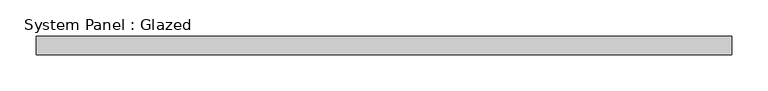
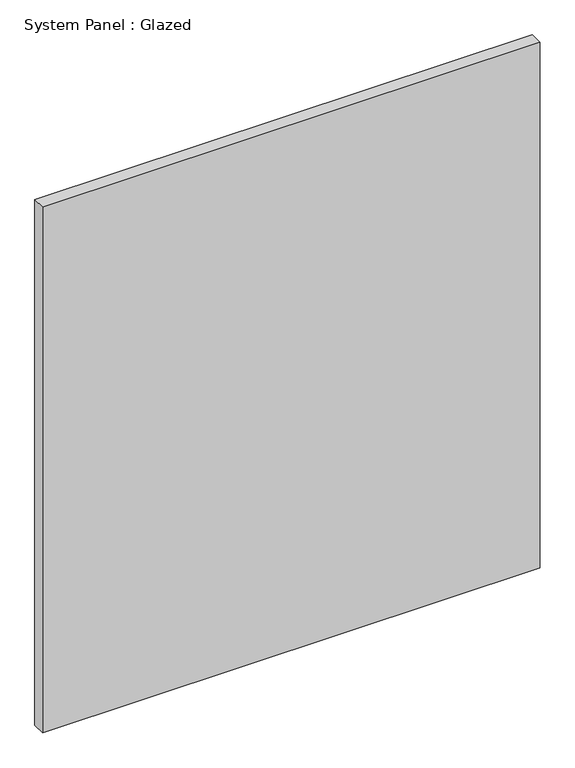
"""IFC4 building model written with IfcOpenShell, lengths in millimetres: plate geometry, System Panel : Glazed."""

from ifc_helpers import new_model, si_unit, origin, origin_with_axes, place, context, project, spatial, polyline, outline, extrude, source, transform, mapped, element, save


def system_panel_glazed_6a711426(model_context):
    return source(origin(), model_context, "Body", "SweptSolid", [
        extrude(outline(polyline([(480.1967538, -44.45), (-480.1967538, -44.45), (-480.1967538, -19.05), (480.1967538, -19.05), (480.1967538, -44.45)])), origin_with_axes(), (0.0, 0.0, 1.0), 1072.3413496),
    ])


if __name__ == "__main__":
    model = new_model("IFC4")
    model_context = context("Model", 3, world=origin())
    ifc_project = project(units=[si_unit("LENGTHUNIT", "METRE", prefix="MILLI")], contexts=[model_context])
    site = spatial("IfcSite", under=ifc_project)
    building = spatial("IfcBuilding", under=site)
    placement = place(None, origin())
    system_panel_glazed_shape = system_panel_glazed_6a711426(model_context)
    element("IfcPlate", 1, ObjectType="System Panel : Glazed", at=placement, inside=building, context=model_context, shape_type="MappedRepresentation", body=[
        mapped(system_panel_glazed_shape, transform((0.0, 0.0, 0.0), x_axis=(1.0, 0.0, 0.0), y_axis=(0.0, 1.0, 0.0), z_axis=(0.0, 0.0, 1.0))),
    ])
    save(model, "model.ifc")

# Revit data of these elements
# Type "System Panel : Glazed"
#   Construction Type Id = "GSP4R"
#   Analytic Construction = "1/8 in Pilkington single glazing"
#   Visual Light Transmittance = 0.9
#   Solar Heat Gain Coefficient = 0.86
#   Heat Transfer Coefficient (U) = 1.18115 BTU/(h·ft²·°F)
#   Define Thermal Properties by = 1
# Element 1 (IfcPlate, "System Panel : Glazed")
#   Materials on its faces: "Glass"
# Materials
#   "Glass": class "Glass", colour RGB 0 128 192, transparency 0.75, Description = "Soda Lime Glass", Cost = 0
